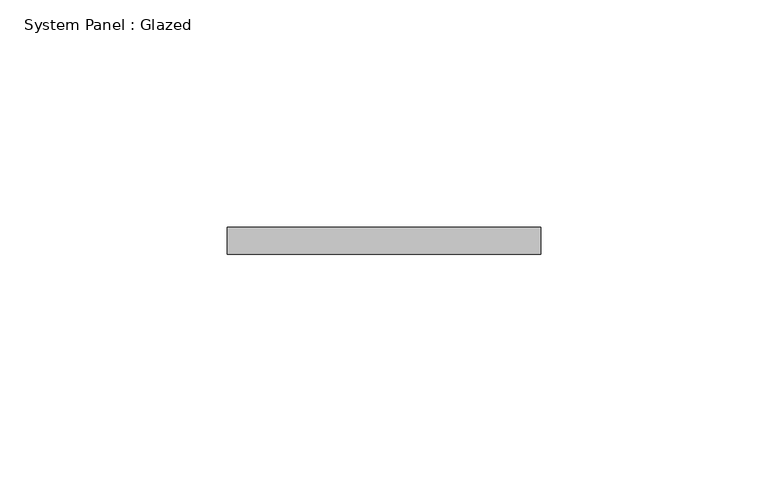
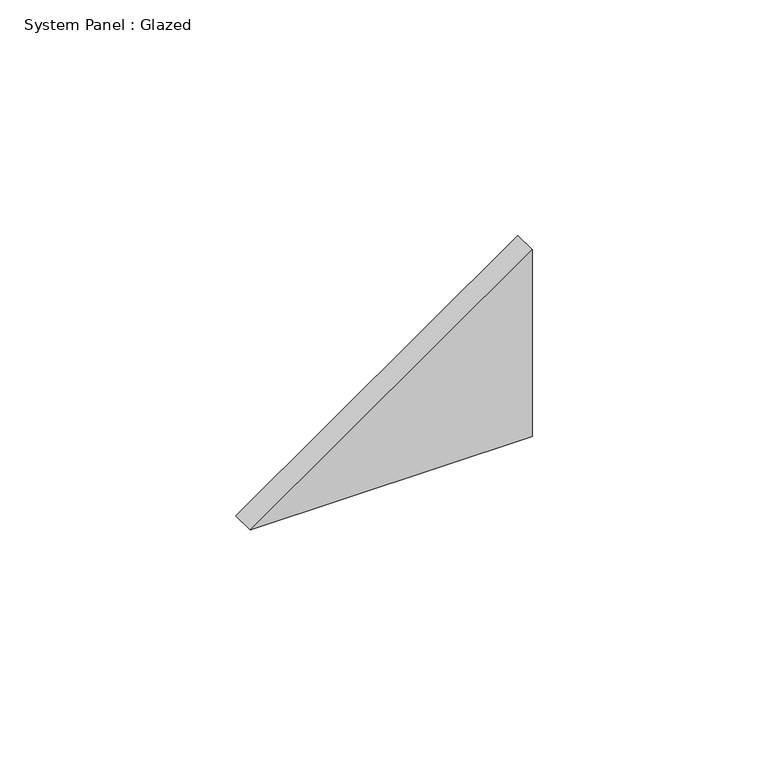
"""IFC4 building model written with IfcOpenShell, lengths in millimetres: plate geometry, System Panel : Glazed."""

from ifc_helpers import new_model, si_unit, frame, origin, place, context, project, spatial, polyline, outline, extrude, source, transform, mapped, element, save


def system_panel_glazed_a9c2f29e(model_context):
    return source(origin(), model_context, "Body", "SweptSolid", [
        extrude(outline(polyline([(0.0, -34.5169591), (0.0, 34.5169591), (48.3380699, 34.5169591), (0.0, -34.5169591)])), frame((0.0, 34.0, 0.0), z_axis=(0.0, 1.0, 0.0), x_axis=(0.0, 0.0, 1.0)), (0.0, 0.0, 1.0), 6.0),
    ])


if __name__ == "__main__":
    model = new_model("IFC4")
    model_context = context("Model", 3, world=origin())
    ifc_project = project(units=[si_unit("LENGTHUNIT", "METRE", prefix="MILLI")], contexts=[model_context])
    site = spatial("IfcSite", under=ifc_project)
    building = spatial("IfcBuilding", under=site)
    placement = place(None, origin())
    system_panel_glazed_shape = system_panel_glazed_a9c2f29e(model_context)
    element("IfcPlate", 1, ObjectType="System Panel : Glazed", at=placement, inside=building, context=model_context, shape_type="MappedRepresentation", body=[
        mapped(system_panel_glazed_shape, transform((0.0, 0.0, 0.0), x_axis=(1.0, 0.0, 0.0), y_axis=(0.0, 1.0, 0.0), z_axis=(0.0, 0.0, 1.0))),
    ])
    save(model, "model.ifc")

# Revit data of these elements
# Type "System Panel : Glazed"
#   Construction Type Id = "GSP4R"
#   Analytic Construction = "1/8 in Pilkington single glazing"
#   Visual Light Transmittance = 0.9
#   Solar Heat Gain Coefficient = 0.86
#   Heat Transfer Coefficient (U) = 6.7069 W/(m²·K)
#   Define Thermal Properties by = 1
# Element 1 (IfcPlate, "System Panel : Glazed")
#   Materials on its faces: "Default New Material(6)"
# Materials
#   "Default New Material(6)": class "Generic", colour RGB 191 25 25, transparency 0.9, Cost = 0
